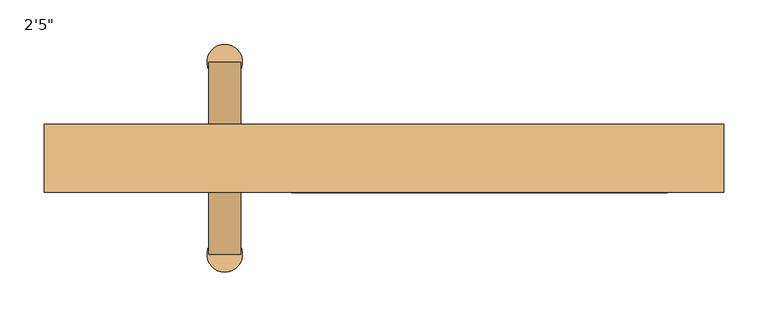
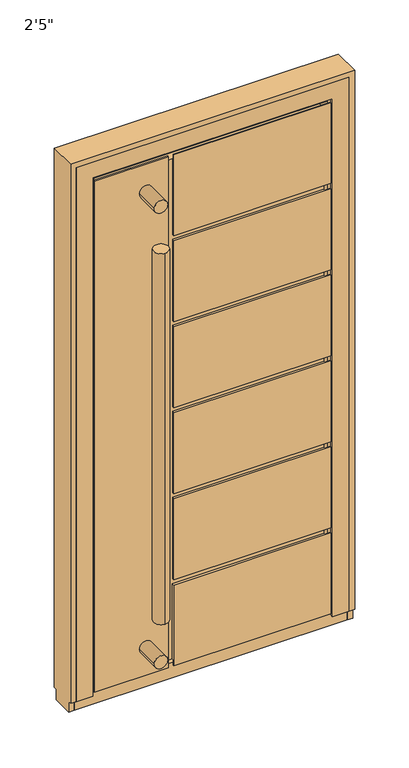
"""IFC4 building model written with IfcOpenShell, lengths in millimetres: door geometry."""

from ifc_helpers import new_model, si_unit, point, frame, frame_2d, origin, place, context, project, spatial, circle_curve, trimmed, segment, composite_curve, outline, extrude, faceted_brep, source, transform, mapped, element, save


def door_dc81b0c5(model_context):
    return source(origin(), model_context, "Body", "SolidModel", [
        extrude(outline(composite_curve([segment(trimmed(circle_curve(frame_2d((-179.75, 90.8003001)), 20.0), [point((-179.75, 70.8003001))], [point((-179.75, 110.8003001))], False, "CARTESIAN"), True, "CONTINUOUS"), segment(trimmed(circle_curve(frame_2d((-179.75, 90.8003001)), 20.0), [point((-179.75, 110.8003001))], [point((-179.75, 70.8003001))], False, "CARTESIAN"), True, "CONTINUOUS")], self_intersect=False)), frame((0.0, 0.0, 210.0000003), z_axis=(0.0, 0.0, 1.0), x_axis=(1.0, 0.0, 0.0)), (0.0, 0.0, 1.0), 1059.0),
        extrude(outline(composite_curve([segment(trimmed(circle_curve(frame_2d((-179.75, -126.2003001)), 20.0), [point((-179.75, -146.2003001))], [point((-179.75, -106.2003001))], False, "CARTESIAN"), True, "CONTINUOUS"), segment(trimmed(circle_curve(frame_2d((-179.75, -126.2003001)), 20.0), [point((-179.75, -106.2003001))], [point((-179.75, -146.2003001))], False, "CARTESIAN"), True, "CONTINUOUS")], self_intersect=False)), frame((0.0, 0.0, 210.0000003), z_axis=(0.0, 0.0, 1.0), x_axis=(1.0, 0.0, 0.0)), (0.0, 0.0, 1.0), 1059.0),
        extrude(outline(composite_curve([segment(trimmed(circle_curve(frame_2d((89.5000003, -179.75)), 18.0), [point((89.5000003, -197.75))], [point((89.5000003, -161.75))], False, "CARTESIAN"), True, "CONTINUOUS"), segment(trimmed(circle_curve(frame_2d((89.5000003, -179.75)), 18.0), [point((89.5000003, -161.75))], [point((89.5000003, -197.75))], False, "CARTESIAN"), True, "CONTINUOUS")], self_intersect=False)), frame((0.0, -126.2, 0.0), z_axis=(0.0, 1.0, 0.0), x_axis=(0.0, 0.0, 1.0)), (0.0, 0.0, 1.0), 217.0),
        extrude(outline(composite_curve([segment(trimmed(circle_curve(frame_2d((1389.5000003, -179.75)), 18.0), [point((1389.5000003, -197.75))], [point((1389.5000003, -161.75))], False, "CARTESIAN"), True, "CONTINUOUS"), segment(trimmed(circle_curve(frame_2d((1389.5000003, -179.75)), 18.0), [point((1389.5000003, -161.75))], [point((1389.5000003, -197.75))], False, "CARTESIAN"), True, "CONTINUOUS")], self_intersect=False)), frame((0.0, -126.2, 0.0), z_axis=(0.0, 1.0, 0.0), x_axis=(0.0, 0.0, 1.0)), (0.0, 0.0, 1.0), 217.0),
        faceted_brep([(-104.75, 13.8, 255.666667), (294.75, 13.8, 255.666667), (294.75, 13.8, 240.666667), (-104.75, 13.8, 240.666667), (-104.75, 13.8, 35.0), (-119.75, 13.8, 35.0), (-119.75, 13.8, 1444.0000003), (-104.75, 13.8, 1444.0000003), (-104.75, 13.8, 1238.3333337), (294.75, 13.8, 1238.3333337), (294.75, 13.8, 1223.3333337), (-104.75, 13.8, 1223.3333337), (-104.75, 13.8, 992.666667), (294.75, 13.8, 992.666667), (294.75, 13.8, 977.666667), (-104.75, 13.8, 977.666667), (-104.75, 13.8, 747.0000004), (294.75, 13.8, 747.0000004), (294.75, 13.8, 732.0000004), (-104.75, 13.8, 732.0000004), (-104.75, 13.8, 501.3333337), (294.75, 13.8, 501.3333337), (294.75, 13.8, 486.3333337), (-104.75, 13.8, 486.3333337), (-104.75, 20.8, 486.3333337), (-104.75, 20.8, 255.666667), (294.75, 20.8, 486.3333337), (294.75, 11.7997698, 1444.0000003), (294.75, 11.7997698, 35.0), (294.75, 18.8020472, 35.0), (294.75, 18.8020472, 24.0), (294.75, 20.8, 24.0), (294.75, 20.8, 240.666667), (294.75, 20.8, 255.666667), (294.75, 20.8, 501.3333337), (294.75, 20.8, 732.0000004), (294.75, 20.8, 747.0000004), (294.75, 20.8, 977.666667), (294.75, 20.8, 992.666667), (294.75, 20.8, 1223.3333337), (294.75, 20.8, 1238.3333337), (294.75, 20.8, 1444.0000003), (-104.75, 20.8, 501.3333337), (-104.75, 20.8, 732.0000004), (-104.75, 20.8, 747.0000004), (-104.75, 20.8, 977.666667), (-119.75, 18.8020472, 35.0), (-119.75, 18.8020472, 24.0), (-119.75, 20.8, 24.0), (-119.75, 20.8, 1444.0000003), (-294.75, 11.7997698, 35.0), (-294.75, 18.8020472, 35.0), (-104.75, 18.8020472, 35.0), (-104.75, 20.8, 240.666667), (-104.75, 20.8, 24.0), (-104.75, 18.8020472, 24.0), (-294.75, 18.8020472, 24.0), (-294.75, 20.8, 24.0), (-294.75, 20.8, 1444.0000003), (-104.75, 20.8, 992.666667), (-104.75, 20.8, 1223.3333337), (-104.75, 20.8, 1238.3333337), (-104.75, 20.8, 1444.0000003), (319.75, -56.2, 10.0000003), (-104.75, -56.2, 10.0000003), (-104.75, -53.2, 10.0000003), (319.75, -53.2, 10.0000003), (-319.75, -53.2, 10.0000003), (-119.75, -53.2, 10.0000003), (-119.75, -56.2, 10.0000003), (-319.75, -56.2, 10.0000003), (319.75, -56.2, 255.666667), (319.75, -53.2, 255.666667), (319.75, -53.2, 486.3333337), (319.75, -56.2, 486.3333337), (319.75, -56.2, 747.0000004), (319.75, -53.2, 747.0000004), (319.75, -53.2, 977.666667), (319.75, -56.2, 977.666667), (319.75, -56.2, 501.3333337), (319.75, -53.2, 501.3333337), (319.75, -53.2, 732.0000004), (319.75, -56.2, 732.0000004), (319.75, -56.2, 992.666667), (319.75, -53.2, 992.666667), (319.75, -53.2, 1223.3333337), (319.75, -56.2, 1223.3333337), (319.75, -56.2, 1469.0000003), (319.75, -56.2, 1238.3333337), (319.75, -53.2, 1238.3333337), (319.75, -53.2, 1469.0000003), (319.75, -53.2, 240.666667), (319.75, -56.2, 240.666667), (-104.75, -53.2, 25.5), (304.25, -53.2, 25.5), (304.25, -53.2, 240.666667), (304.25, -53.2, 255.666667), (304.25, -53.2, 486.3333337), (304.25, -53.2, 747.0000004), (304.25, -53.2, 977.666667), (304.25, -53.2, 501.3333337), (304.25, -53.2, 732.0000004), (-304.25, -53.2, 25.5), (-119.75, -53.2, 25.5), (-319.75, -53.2, 1469.0000003), (-119.75, -53.2, 1469.0000003), (-119.75, -53.2, 1453.5000003), (-304.25, -53.2, 1453.5000003), (304.25, -53.2, 992.666667), (304.25, -53.2, 1223.3333337), (304.25, -53.2, 1238.3333337), (304.25, -53.2, 1453.5000003), (-104.75, -53.2, 1453.5000003), (-104.75, -53.2, 1469.0000003), (-104.75, -49.2, 240.666667), (-104.75, -49.2, 25.5), (-104.75, -56.2, 240.666667), (-119.75, -56.2, 1469.0000003), (-319.75, -56.2, 1469.0000003), (-104.75, -56.2, 486.3333337), (-104.75, -56.2, 255.666667), (-104.75, -56.2, 977.666667), (-104.75, -56.2, 747.0000004), (-104.75, -56.2, 732.0000004), (-104.75, -56.2, 501.3333337), (-104.75, -56.2, 1223.3333337), (-104.75, -56.2, 992.666667), (-104.75, -56.2, 1469.0000003), (-104.75, -56.2, 1238.3333337), (-119.75, -49.2, 1453.5000003), (-119.75, -49.2, 25.5), (-294.75, 11.7997698, 1444.0000003), (304.25, 11.7997698, 1453.5000003), (304.25, 11.7997698, 25.5), (-304.25, 11.7997698, 25.5), (-304.25, 11.7997698, 1453.5000003), (304.25, -49.2, 1238.3333337), (304.25, -49.2, 1223.3333337), (304.25, -49.2, 992.666667), (304.25, -49.2, 977.666667), (304.25, -49.2, 747.0000004), (304.25, -49.2, 732.0000004), (304.25, -49.2, 501.3333337), (304.25, -49.2, 486.3333337), (304.25, -49.2, 255.666667), (304.25, -49.2, 240.666667), (-104.75, -49.2, 1223.3333337), (-104.75, -49.2, 1238.3333337), (-104.75, -49.2, 1453.5000003), (-104.75, -49.2, 255.666667), (-104.75, -49.2, 486.3333337), (-104.75, -49.2, 501.3333337), (-104.75, -49.2, 732.0000004), (-104.75, -49.2, 747.0000004), (-104.75, -49.2, 977.666667), (-104.75, -49.2, 992.666667)], [[[0, 1, 2, 3, 4, 5, 6, 7, 8, 9, 10, 11, 12, 13, 14, 15, 16, 17, 18, 19, 20, 21, 22, 23]], [[23, 24, 25, 0]], [[23, 22, 26, 24]], [[27, 28, 29, 30, 31, 32, 2, 1, 33, 26, 22, 21, 34, 35, 18, 17, 36, 37, 14, 13, 38, 39, 10, 9, 40, 41]], [[42, 34, 21, 20]], [[19, 43, 42, 20]], [[19, 18, 35, 43]], [[44, 36, 17, 16]], [[15, 45, 44, 16]], [[5, 46, 47, 48, 49, 6]], [[28, 50, 51, 46, 5, 4, 52, 29]], [[53, 54, 55, 52, 4, 3]], [[3, 2, 32, 53]], [[25, 33, 1, 0]], [[29, 52, 55, 30]], [[56, 47, 46, 51]], [[30, 55, 54, 31]], [[57, 48, 47, 56]], [[36, 44, 45, 37]], [[34, 42, 43, 35]], [[33, 25, 24, 26]], [[54, 53, 32, 31]], [[58, 49, 48, 57]], [[38, 59, 60, 39]], [[41, 40, 61, 62]], [[63, 64, 65, 66]], [[67, 68, 69, 70]], [[71, 72, 73, 74]], [[75, 76, 77, 78]], [[79, 80, 81, 82]], [[83, 84, 85, 86]], [[87, 88, 89, 90]], [[66, 91, 92, 63]], [[65, 93, 94, 95, 91, 66]], [[72, 96, 97, 73]], [[76, 98, 99, 77]], [[80, 100, 101, 81]], [[102, 103, 68, 67, 104, 105, 106, 107]], [[84, 108, 109, 85]], [[90, 89, 110, 111, 112, 113]], [[114, 115, 93, 65, 64, 116]], [[70, 69, 117, 118]], [[63, 92, 116, 64]], [[74, 119, 120, 71]], [[78, 121, 122, 75]], [[82, 123, 124, 79]], [[86, 125, 126, 83]], [[87, 127, 128, 88]], [[70, 118, 104, 67]], [[129, 106, 105, 117, 69, 68, 103, 130]], [[58, 57, 56, 51, 50, 131]], [[132, 133, 134, 135], [131, 50, 28, 27]], [[111, 110, 136, 137, 109, 108, 138, 139, 99, 98, 140, 141, 101, 100, 142, 143, 97, 96, 144, 145, 95, 94, 133, 132]], [[94, 93, 115, 130, 103, 102, 134, 133]], [[135, 134, 102, 107]], [[146, 137, 136, 147, 148, 129, 130, 115, 114, 145, 144, 149, 150, 143, 142, 151, 152, 141, 140, 153, 154, 139, 138, 155]], [[153, 122, 121, 154]], [[153, 140, 98, 76, 75, 122]], [[123, 82, 81, 101, 141, 152]], [[151, 124, 123, 152]], [[151, 142, 100, 80, 79, 124]], [[119, 74, 73, 97, 143, 150]], [[149, 120, 119, 150]], [[149, 144, 96, 72, 71, 120]], [[116, 92, 91, 95, 145, 114]], [[15, 14, 37, 45]], [[59, 38, 13, 12]], [[11, 60, 59, 12]], [[11, 10, 39, 60]], [[61, 40, 9, 8]], [[8, 7, 62, 61]], [[125, 86, 85, 109, 137, 146]], [[128, 127, 113, 112, 148, 147]], [[121, 78, 77, 99, 139, 154]], [[155, 138, 108, 84, 83, 126]], [[155, 126, 125, 146]], [[147, 136, 110, 89, 88, 128]], [[90, 113, 127, 87]], [[118, 117, 105, 104]], [[132, 135, 107, 106, 129, 148, 112, 111]], [[27, 41, 62, 7, 6, 49, 58, 131]]]),
        faceted_brep([(-368.3, -56.2, 0.0), (-368.3, -47.1997571, 0.0), (-323.8, -47.1997571, 0.0), (-323.8, -56.2, 0.0), (-314.3, 16.2999958, 0.0), (-314.3, 11.8, 0.0), (-368.3, 11.8, 0.0), (-368.3, 20.8, 0.0), (-298.8, 20.8, 0.0), (-298.8, 16.2999958, 0.0), (368.3, 20.8, 0.0), (368.3, 11.8, 0.0), (314.3, 11.8, 0.0), (314.3, 16.2999958, 0.0), (298.8, 16.2999958, 0.0), (298.8, 20.8, 0.0), (323.8, -47.1997571, 0.0), (368.3, -47.1997571, 0.0), (368.3, -56.2, 0.0), (323.8, -56.2, 0.0), (-368.3, 11.8, -30.0), (-368.3, -47.1997571, -30.0), (-368.3, -56.2, 1524.0), (-368.3, 20.8, 1524.0), (-323.8, -56.2, 1479.5), (323.8, -56.2, 1479.5), (368.3, -56.2, 1524.0), (368.3, 20.8, 1524.0), (368.3, -47.1997571, -30.0), (368.3, 11.8, -30.0), (298.8, 20.8, 1454.5), (-298.8, 20.8, 1454.5), (-314.3, -47.2, 1470.0), (-314.3, -47.2, 14.5), (-314.3, 11.8, 14.5), (-314.3, 16.2999958, 1470.0), (314.3, 16.2999958, 1470.0), (314.3, -47.2, 1470.0), (314.3, 11.8, 14.5), (314.3, -47.2, 14.5), (-323.8, -47.2, 1479.5), (323.8, -47.2, 1479.5), (-298.8, 16.2999958, 1454.5), (298.8, 16.2999958, 1454.5)], [[[0, 1, 2, 3]], [[4, 5, 6, 7, 8, 9]], [[10, 11, 12, 13, 14, 15]], [[16, 17, 18, 19]], [[7, 6, 20, 21, 1, 0, 22, 23]], [[3, 24, 25, 19, 18, 26, 22, 0]], [[22, 26, 27, 23]], [[18, 17, 28, 29, 11, 10, 27, 26]], [[7, 23, 27, 10, 15, 30, 31, 8]], [[32, 33, 34, 5, 4, 35]], [[35, 36, 37, 32]], [[36, 13, 12, 38, 39, 37]], [[40, 24, 3, 2]], [[16, 41, 40, 2, 1, 21, 28, 17], [37, 39, 33, 32]], [[9, 42, 43, 14, 13, 36, 35, 4]], [[8, 31, 42, 9]], [[24, 40, 41, 25]], [[30, 43, 42, 31]], [[19, 25, 41, 16]], [[14, 43, 30, 15]], [[20, 6, 5, 34, 38, 12, 11, 29]], [[39, 38, 34, 33]], [[20, 29, 28, 21]]]),
        faceted_brep([(-368.3, -47.2, -30.0), (-383.3, -47.2, -30.0), (-383.3, 11.8, -30.0), (-368.3, 11.8, -30.0), (-368.3, -56.2, 1524.0), (-368.3, -56.2, 0.0), (-368.3, -47.2, 0.0), (-368.3, 11.8, 0.0), (-368.3, 20.8, 0.0), (-368.3, 20.8, 1524.0), (-383.3, 11.8, 0.0), (383.3, 11.8, 0.0), (383.3, 11.8, -30.0), (368.3, 11.8, -30.0), (368.3, 11.8, 0.0), (-383.3, 20.8, 1539.0), (-383.3, 20.8, 0.0), (-383.3, -47.2, 0.0), (-383.3, -56.2, 0.0), (-383.3, -56.2, 1539.0), (368.3, -47.2, 0.0), (368.3, -47.2, -30.0), (383.3, -47.2, -30.0), (383.3, -47.2, 0.0), (368.3, 20.8, 1524.0), (368.3, 20.8, 0.0), (368.3, -56.2, 0.0), (368.3, -56.2, 1524.0), (383.3, -56.2, 0.0), (383.3, -56.2, 1539.0), (383.3, 20.8, 0.0), (383.3, 20.8, 1539.0)], [[[0, 1, 2, 3]], [[4, 5, 6, 0, 3, 7, 8, 9]], [[7, 3, 2, 10]], [[11, 12, 13, 14]], [[15, 16, 10, 2, 1, 17, 18, 19]], [[17, 1, 0, 6]], [[20, 21, 22, 23]], [[24, 25, 14, 13, 21, 20, 26, 27]], [[27, 26, 28, 29, 19, 18, 5, 4]], [[6, 5, 18, 17]], [[23, 28, 26, 20]], [[22, 21, 13, 12]], [[10, 16, 8, 7]], [[14, 25, 30, 11]], [[9, 8, 16, 15, 31, 30, 25, 24]], [[29, 28, 23, 22, 12, 11, 30, 31]], [[9, 24, 27, 4]], [[19, 29, 31, 15]]]),
    ])


if __name__ == "__main__":
    model = new_model("IFC4")
    model_context = context("Model", 3, world=origin())
    ifc_project = project(units=[si_unit("LENGTHUNIT", "METRE", prefix="MILLI")], contexts=[model_context])
    site = spatial("IfcSite", under=ifc_project)
    building = spatial("IfcBuilding", under=site)
    placement = place(None, origin())
    door_shape = door_dc81b0c5(model_context)
    element("IfcDoor", 1, ObjectType="2'5\"", at=placement, inside=building, context=model_context, shape_type="MappedRepresentation", body=[
        mapped(door_shape, transform((0.0, 0.0, 0.0), x_axis=(1.0, 0.0, 0.0), y_axis=(0.0, 1.0, 0.0), z_axis=(0.0, 0.0, 1.0))),
    ])
    save(model, "model.ifc")

# Revit data of these elements
# Type "2'5\""
#   Type Mark = "9"
#   Water resistance = "up to Class E900, EN 12208:2001"
#   Uniclass2015Version = "v1.21"
#   Uniclass2015Reference = "Ss_25_30_20_30"
#   Uniclass2015Description = "Frame and door leaf system"
#   URL = "www.aluprof.com"
#   Type IFC Predefined Type = "USERDEFINED"
#   Right-hand / Left-hand door [instance default] = ""
#   Resistance to wind load = "up to Class C5/B5, EN 12210:2001"
#   Insert type = "ST"
#   Hardware [instance default] = ""
#   Product page = "https://aluprof.com/en/architects/offer/window-and-door-systems/panel-doors#visualisation"
#   Operation = "SinglePanelOutwardOpening"
#   Opening type = "Outward"
#   NBSReference = "25-50-20/125"
#   NBSDescription = "Frame and door leaf system"
#   Important = "The actual acceptable construction dimensions are dependent on the selection of profiles and hardware, glazing type, construction weight and the construction’s operating conditions. These should be determined by a suitably qualified person, and using ALUPROF’s calculation software"
#   IfcExportType = "USERDEFINED"
#   IfcExportAs = "IfcDoorType"
#   Handle type [instance default] = ""
#   Manufacturer = "ALUPROF SA"
#   Export Type to IFC As = "IfcDoorType"
#   Door sill type [instance default] = ""
#   Description = "External single-leaf panel door outward opening"
#   Model = "MB-86 ST Panel Door AD07"
#   Content of the recyclate in the material = "69.2%"
#   COBie.Type.WarrantyDurationParts = ""
#   COBie.Type.Name = ""
#   COBie.Type.Manufacturer = "ALUPROF SA"
#   COBie.Space.Name = ""
#   COBie.Floor.Name = ""
#   COBie.Facility.Name = ""
#   COBie.CreatedOn = ""
#   COBie.Component.WarrantyStartDate = ""
#   COBie.Component.Name = "MB-86 ST Panel Door AD07"
#   Burglar resistance = "RC2"
#   Air permeability = "up to Class 4, EN 12207:2001"
#   Width of the active leaf = 2' - 1.17717"
#   Placement in wall = 0' - 0.7874"
#   Thickness = 0' - 3.0315"
#   Height of the opening sash = 4' - 9.44094"
#   Handle Offset = 3' - 5.33858"
#   Rough Height = 5' - 2.40945"
#   Rough Width = 2' - 6.1811"
#   Height = 5' - 0"
#   Width = 2' - 5"
#   Construction depth = 0' - 3.0315"
#   Clear opening width = 1' - 8.94882"
#   Clear opening height = 4' - 8.47638"
#   Height of the array = 0' - 9.08136"
#   Schedule No. [instance default] = 1
#   Handrail [instance default] = yes
#   IsExternal = yes
#   Handle [instance default] = no
#   Door closer [instance default] = no
#   Function = 1
#   COBie.Type = yes
#   COBie = yes
#   Access control [instance default] = no
#   Panel = element 346771
#   Wall Closure = (empty or 0)
